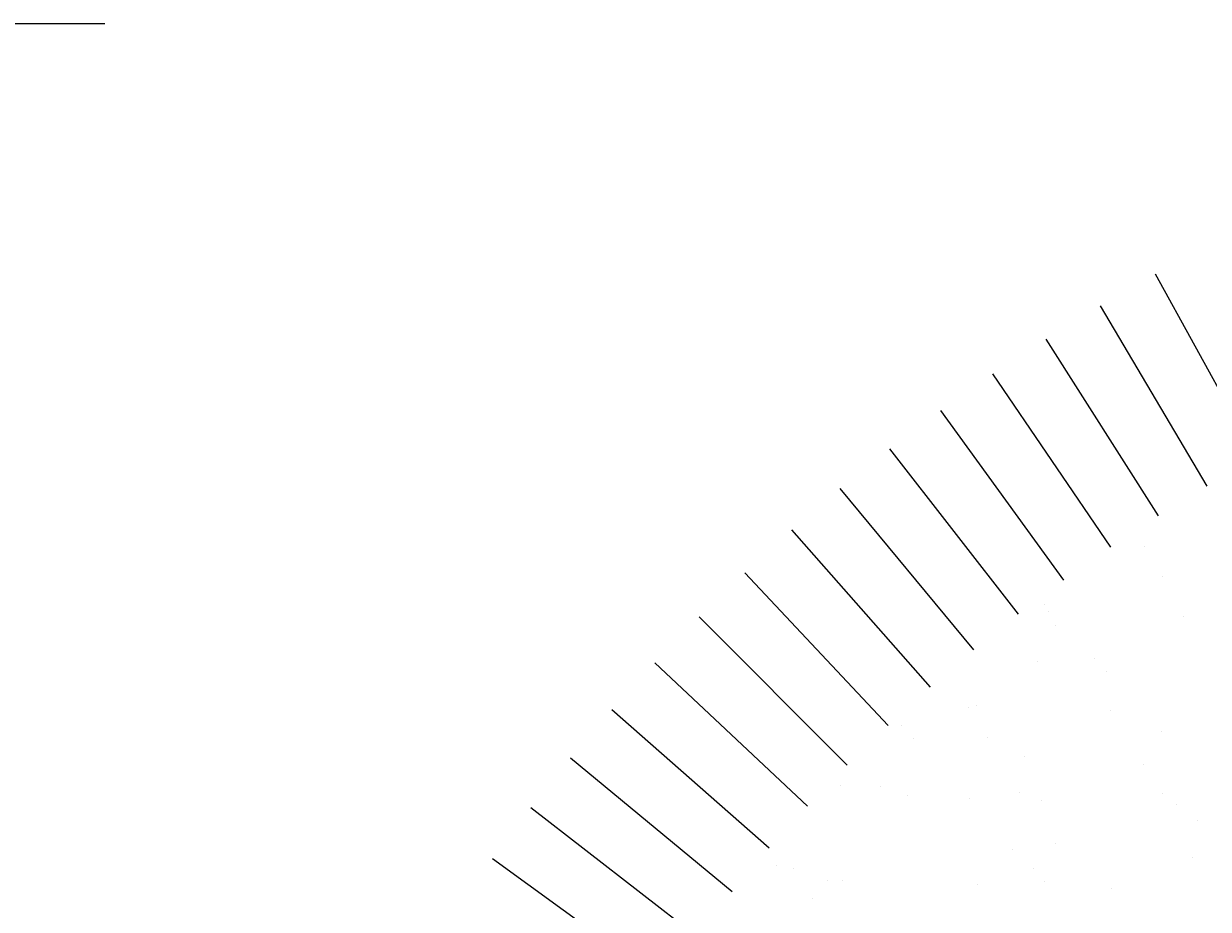
# Model space of a CAD drawing. Units: millimetres. Extents: x -857 to 54106, y -13666 to 13947.
# Tile 37 of 41: x 30856 to 31622, y 10517 to 11089. Entities that reach past the tile are written whole.
import ezdxf

# ---------------------------------------------------------------- set-up
doc = ezdxf.new("R2010")
doc.units = ezdxf.units.MM
doc.layers.add('A-ANNO-DIMS', color=2, linetype='Continuous', lineweight=18)
doc.layers.add('A-FURN', color=21, linetype='Continuous', lineweight=18)
doc.layers.add('A-HT', color=15, linetype='Continuous')
doc.styles.get("Standard").update_dxf_attribs({"font": 'arial.ttf'})
doc.dimstyles.new('ISO-25', dxfattribs={"dimtxt": 2.5, "dimasz": 2.5, "dimexe": 1.25, "dimexo": 0.625, "dimtad": 1, "dimtxsty": 'Standard', "dimcen": 2.5, "dimadec": 0, "dimazin": 0, "dimtfac": 1, "dimtmove": 0, "dimatfit": 3, "dimfxl": 1, "dimarcsym": 0})

# ---------------------------------------------------------------- blocks, each defined once
blk = doc.blocks.new('*X18')
at = {"color": 0}
for p, q in [((1.15267, 2.5197), (1.15267, 2.5197)), ((1.15506, 2.50778), (1.15506, 2.50778)), ((1.17615, 2.49435), (1.17615, 2.49435)), ((1.16301, 2.48335), (1.16301, 2.48335)), ((1.09509, 2.47441), (1.09509, 2.47441)), ((1.16304, 2.47256), (1.16304, 2.47256)), ((1.09635, 2.44571), (1.09635, 2.44571)), ((1.05213, 2.43021), (1.05213, 2.43021)), ((1.10274, 2.42629), (1.10274, 2.42629)), ((1.06135, 2.42177), (1.06135, 2.42177)), ((1.03828, 2.37683), (1.03828, 2.37683)), ((1.03974, 2.38229), (1.03974, 2.38229)), ((1.10485, 2.38191), (1.10485, 2.38191)), ((1.16619, 2.37622), (1.16619, 2.37622)), ((1.06082, 2.36886), (1.06082, 2.36886)), ((1.14119, 2.35102), (1.14119, 2.35102)), ((1.07452, 2.34224), (1.07452, 2.34224)), ((1.10054, 2.34567), (1.10054, 2.34567)), ((1.0066, 2.3333), (1.0066, 2.3333)), ((1.15462, 2.3363), (1.15462, 2.3363)), ((0.96596, 2.32795), (0.96596, 2.32795)), ((0.97085, 2.32509), (0.97085, 2.32509)), ((1.10589, 2.32995), (1.10589, 2.32995)), ((1.16383, 2.32786), (1.16383, 2.32786)), ((0.98102, 2.32022), (0.98102, 2.32022)), ((1.13673, 2.3205), (1.13673, 2.3205)), ((1.00431, 2.29242), (1.00431, 2.29242)), ((1.01353, 2.28398), (1.01353, 2.28398)), ((1.04143, 2.28049), (1.04143, 2.28049)), ((1.16934, 2.27988), (1.16934, 2.27988)), ((0.92441, 2.2568), (0.92441, 2.2568)), ((1.08012, 2.25709), (1.08012, 2.25709)), ((0.9455, 2.24337), (0.9455, 2.24337)), ((1.05702, 2.24412), (1.05702, 2.24412)), ((1.1012, 2.24365), (1.1012, 2.24365)), ((1.10904, 2.23361), (1.10904, 2.23361)), ((0.974, 2.22875), (0.974, 2.22875)), ((1.14664, 2.22228), (1.14664, 2.22228)), ((1.12062, 2.21885), (1.12062, 2.21885))]:
    blk.add_line(p, q, dxfattribs=at)
blk = doc.blocks.new('A$C6796526C')
at = {"layer": 'A-HT'}
for p, q in [((0.3108, 0.82372), (0.17936, 0.75146)), ((0.33104, 0.78825), (0.20192, 0.71189)), ((0.35237, 0.75343), (0.22572, 0.67305)), ((0.3748, 0.71929), (0.25073, 0.63498)), ((0.39828, 0.68588), (0.27693, 0.59771)), ((0.4228, 0.65322), (0.30428, 0.56128)), ((0.44833, 0.62135), (0.33276, 0.52574)), ((0.47486, 0.59029), (0.36234, 0.4911)), ((0.50234, 0.56009), (0.393, 0.45741)), ((0.53076, 0.53076), (0.4247, 0.4247)), ((0.56009, 0.50234), (0.45741, 0.393)), ((0.59029, 0.47486), (0.4911, 0.36234)), ((0.62135, 0.44833), (0.52574, 0.33276)), ((0.65322, 0.4228), (0.56128, 0.30428)), ((0.68588, 0.39828), (0.59771, 0.27693))]:
    blk.add_line(p, q, dxfattribs=at)
at = {"layer": 'A-HT', "extrusion": (0, 0, -1), "zscale": -1, "rotation": 180}
blk.add_blockref('*X18', (0.55, 3), dxfattribs=at)
blk = doc.blocks.new('*D48')
at = {"layer": 'A-ANNO-DIMS', "color": 0, "lineweight": -2, "transparency": 16777216}
for p, q in [((30908.63, 11089.46), (30501.38, 11089.46)), ((30502.63, 11086.96), (30502.63, 8471.5)), ((30908.63, 8469), (30501.38, 8469))]:
    blk.add_line(p, q, dxfattribs=at)
at = {"layer": 'A-ANNO-DIMS', "color": 0, "transparency": 16777216}
for points in [[(30502.21, 11086.96), (30503.05, 11086.96), (30502.63, 11089.46)], [(30502.21, 8471.5), (30503.05, 8471.5), (30502.63, 8469)]]:
    blk.add_solid(points, dxfattribs=at)
at = {"layer": 'Defpoints', "color": 0, "transparency": 16777216}
for p in [(30909.25, 11089.46), (30502.63, 8469), (30909.25, 8469)]:
    blk.add_point(p, dxfattribs=at)
at = {"layer": 'A-ANNO-DIMS', "color": 0, "transparency": 16777216, "insert": (30500.73, 9779.23), "char_height": 2.5, "attachment_point": 5, "rotation": 90}
blk.add_mtext('2620 TYP.', dxfattribs=at)

msp = doc.modelspace()

# ---------------------------------------------------------------- block references
at = {"layer": 'A-FURN', "xscale": 903.6084929786902, "yscale": 903.6084929786902, "zscale": 903.6084929786902, "rotation": 269.9999999999988}
msp.add_blockref('A$C6796526C', (30909.253, 11089.463), dxfattribs=at)

# ---------------------------------------------------------------- dimensions: what is measured, and where the dimension line sits
at = {"layer": 'A-ANNO-DIMS'}
dim = msp.add_linear_dim(base=(30502.63, 8468.999), p1=(30909.254, 11089.463), p2=(30909.254, 8468.999), angle=270, text='<> TYP.', dimstyle='ISO-25', override={"dimdec": 0, "dimrnd": 0, "dimzin": 0, "dimlunit": 2}, dxfattribs=at)
dim.commit()
dim.dimension.update_dxf_attribs({"geometry": '*D48', "text_midpoint": (30500.728, 9779.231)})

doc.saveas('drawing.dxf')
